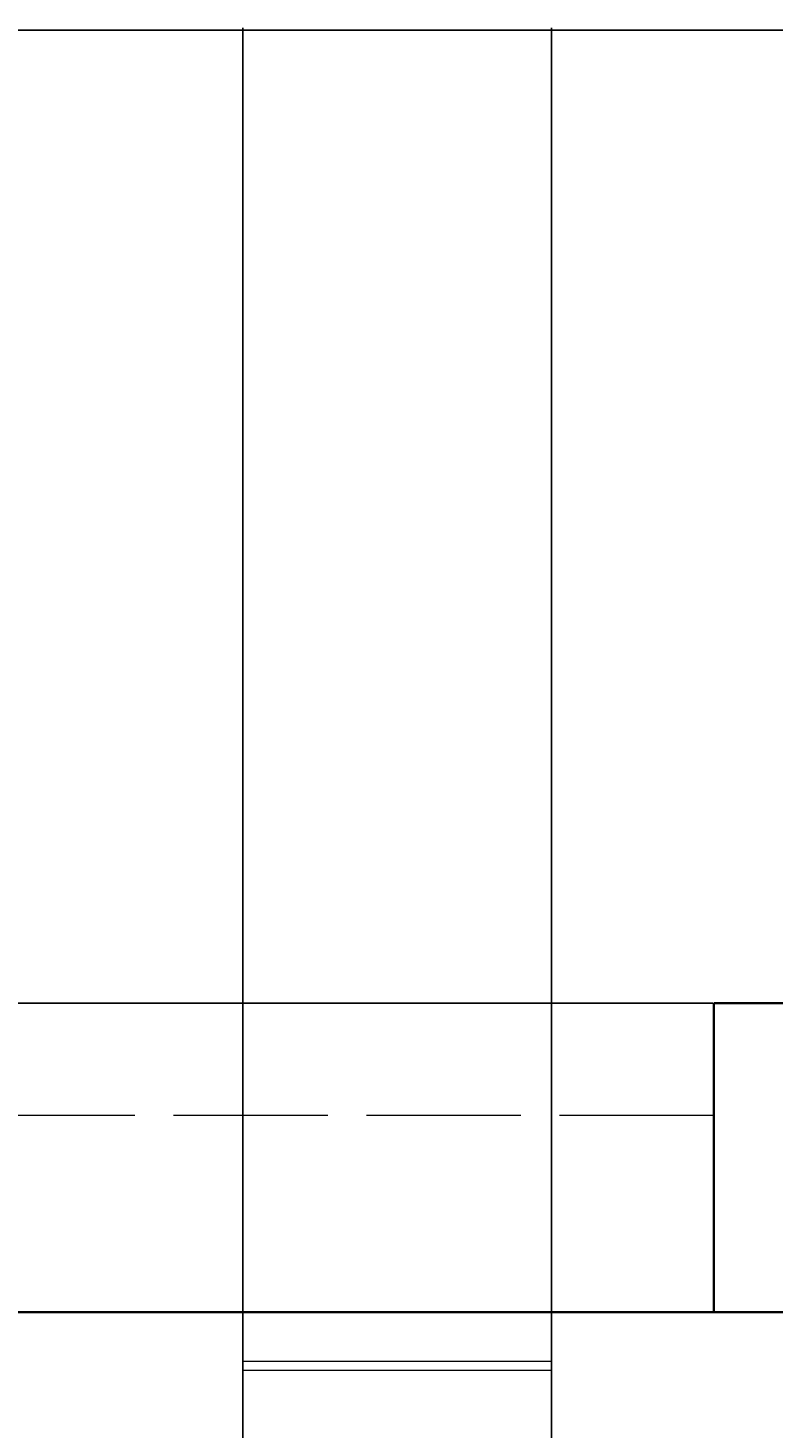
# Model space of a CAD drawing. Units: inches. Extents: x -61 to 1599, y -1316 to 257.
# Tile 142 of 204: x 236 to 294, y 149 to 257. Entities that reach past the tile are written whole.
import ezdxf

# ---------------------------------------------------------------- set-up
doc = ezdxf.new("R2010")
doc.units = ezdxf.units.IN
doc.header["$MEASUREMENT"] = 0
doc.linetypes.add('ACAD_ISO02W100', pattern=[15, 12, -3])
for name, color, linetype, lineweight in [('A-ANNO-DIMS', 2, 'Continuous', 18), ('A-FLOR-OVHD', 203, 'ACAD_ISO02W100', 13), ('WALLS', 4, 'Continuous', 35), ('WINDOWS', 220, 'Continuous', 18)]:
    doc.layers.add(name, color=color, linetype=linetype, lineweight=lineweight)
doc.styles.get("Standard").update_dxf_attribs({"font": 'arial.ttf'})
doc.dimstyles.get("Standard").update_dxf_attribs({"dimtxt": 0.18, "dimasz": 0.18, "dimexe": 0.18, "dimexo": 0.0625, "dimgap": 0.09, "dimtad": 0, "dimtih": 1, "dimtoh": 1, "dimdec": 0, "dimzin": 0, "dimdsep": 46, "dimlunit": 3, "dimtxsty": 'Standard', "dimcen": 0.09, "dimadec": 0, "dimazin": 0, "dimtfac": 1, "dimtdec": 0, "dimtofl": 0, "dimtmove": 0, "dimatfit": 3, "dimfxl": 1, "dimtolj": 1, "dimtzin": 0, "dimarcsym": 0})

# ---------------------------------------------------------------- blocks, each defined once
blk = doc.blocks.new('WIN-24IN')
for p, q in [((0, 4.5), (0, 9)), ((0, 9), (0, 0)), ((24, 9), (24, 0)), ((0, 5.19), (24, 5.19)), ((0, 4.5), (24, 4.5))]:
    blk.add_line(p, q)
blk = doc.blocks.new('*D686')
at = {"layer": 'A-ANNO-DIMS', "color": 0, "lineweight": -2, "transparency": 16777216}
for p, q in [((14.7, 157.74), (14.7, 257.46)), ((14.88, 257.28), (768.35, 257.28)), ((1522.52, 257.28), (769.05, 257.28)), ((1522.7, 157.74), (1522.7, 257.46))]:
    blk.add_line(p, q, dxfattribs=at)
at = {"layer": 'A-ANNO-DIMS', "color": 0, "transparency": 16777216}
for points in [[(14.88, 257.31), (14.88, 257.25), (14.7, 257.28)], [(1522.52, 257.31), (1522.52, 257.25), (1522.7, 257.28)]]:
    blk.add_solid(points, dxfattribs=at)
at = {"layer": 'DEFPOINTS', "color": 0, "transparency": 16777216}
for p in [(1522.7, 257.28), (14.7, 157.68), (1522.7, 157.68)]:
    blk.add_point(p, dxfattribs=at)
at = {"layer": 'A-ANNO-DIMS', "color": 0, "transparency": 16777216, "insert": (768.7, 257.28), "char_height": 0.18, "attachment_point": 5}
blk.add_mtext('\\A1;1508', dxfattribs=at)
blk = doc.blocks.new('*D687')
at = {"layer": 'A-ANNO-DIMS', "color": 0, "lineweight": -2, "transparency": 16777216}
for p, q in [((289.42, 181.68), (-61.08, 181.68)), ((-60.9, 181.5), (-60.9, -528.95)), ((-60.9, -1239.76), (-60.9, -529.32)), ((319.64, -1239.94), (-61.08, -1239.94))]:
    blk.add_line(p, q, dxfattribs=at)
at = {"layer": 'A-ANNO-DIMS', "color": 0, "transparency": 16777216}
for points in [[(-60.93, 181.5), (-60.87, 181.5), (-60.9, 181.68)], [(-60.93, -1239.76), (-60.87, -1239.76), (-60.9, -1239.94)]]:
    blk.add_solid(points, dxfattribs=at)
at = {"layer": 'DEFPOINTS', "color": 0, "transparency": 16777216}
for p in [(289.48, 181.68), (-60.9, -1239.94), (319.7, -1239.94)]:
    blk.add_point(p, dxfattribs=at)
at = {"layer": 'A-ANNO-DIMS', "color": 0, "transparency": 16777216, "insert": (-60.9, -529.13), "char_height": 0.18, "attachment_point": 5}
blk.add_mtext('\\A1;1421.6', dxfattribs=at)
blk = doc.blocks.new('*D701')
at = {"layer": 'A-ANNO-DIMS', "color": 0, "lineweight": -2, "transparency": 16777216}
for p, q in [((215.75, -616.88), (215.75, 257.46)), ((215.93, 257.28), (233.92, 257.28)), ((252.7, 257.28), (234.71, 257.28)), ((252.88, -616.88), (252.88, 257.46))]:
    blk.add_line(p, q, dxfattribs=at)
at = {"layer": 'A-ANNO-DIMS', "color": 0, "transparency": 16777216}
for points in [[(215.93, 257.31), (215.93, 257.25), (215.75, 257.28)], [(252.7, 257.31), (252.7, 257.25), (252.88, 257.28)]]:
    blk.add_solid(points, dxfattribs=at)
at = {"layer": 'DEFPOINTS', "color": 0, "transparency": 16777216}
for p in [(252.88, 257.28), (215.75, -616.94), (252.88, -616.94)]:
    blk.add_point(p, dxfattribs=at)
at = {"layer": 'A-ANNO-DIMS', "color": 0, "transparency": 16777216, "insert": (234.32, 257.28), "char_height": 0.18, "attachment_point": 5}
blk.add_mtext('\\A1;37.13', dxfattribs=at)
blk = doc.blocks.new('*D702')
at = {"layer": 'A-ANNO-DIMS', "color": 0, "lineweight": -2, "transparency": 16777216}
for p, q in [((276.88, -616.88), (276.88, 257.46)), ((277.06, 257.28), (312.21, 257.28)), ((348.14, 257.28), (312.99, 257.28)), ((348.32, -616.88), (348.32, 257.46))]:
    blk.add_line(p, q, dxfattribs=at)
at = {"layer": 'A-ANNO-DIMS', "color": 0, "transparency": 16777216}
for points in [[(277.06, 257.31), (277.06, 257.25), (276.88, 257.28)], [(348.14, 257.31), (348.14, 257.25), (348.32, 257.28)]]:
    blk.add_solid(points, dxfattribs=at)
at = {"layer": 'DEFPOINTS', "color": 0, "transparency": 16777216}
for p in [(348.32, 257.28), (276.88, -616.94), (348.32, -616.94)]:
    blk.add_point(p, dxfattribs=at)
at = {"layer": 'A-ANNO-DIMS', "color": 0, "transparency": 16777216, "insert": (312.6, 257.28), "char_height": 0.18, "attachment_point": 5}
blk.add_mtext('\\A1;71.44', dxfattribs=at)

msp = doc.modelspace()

# ---------------------------------------------------------------- linework, layer by layer
at = {"layer": 'A-FLOR-OVHD'}
msp.add_line((289.4807, 172.9695), (160.8585, 172.9695), dxfattribs=at)
at = {"layer": 'WALLS'}
for p, q in [((289.4807, 157.6771), (289.4807, 181.6771)), ((403.7028, 181.6771), (289.4807, 181.6771)), ((544.7028, 157.6771), (14.7028, 157.6771))]:
    msp.add_line(p, q, dxfattribs=at)

# ---------------------------------------------------------------- block references
at = {"layer": 'WINDOWS'}
msp.add_blockref('WIN-24IN', (252.882, 148.677), dxfattribs=at)

# ---------------------------------------------------------------- dimensions: what is measured, and where the dimension line sits
at = {"layer": 'A-ANNO-DIMS'}
for base, p1, p2, override, picture, middle in [((1522.7028, 257.2771), (14.7028, 157.6771), (1522.7028, 157.6771), {"dimdec": 0, "dimlfac": 1, "dimrnd": 0, "dimzin": 0, "dimdsep": 46, "dimlunit": 2}, '*D686', (768.7028, 257.2771)), ((252.8825, 257.2771), (215.7521, -616.9446), (252.8825, -616.9446), {"dimdec": 2, "dimlfac": 1, "dimrnd": 0, "dimzin": 0, "dimdsep": 46, "dimlunit": 2}, '*D701', (234.3173, 257.2771)), ((348.3201, 257.2771), (276.8825, -616.9446), (348.3201, -616.9446), {"dimdec": 2, "dimlfac": 1, "dimrnd": 0, "dimzin": 0, "dimdsep": 46, "dimlunit": 2}, '*D702', (312.6013, 257.2771))]:
    dim = msp.add_linear_dim(base=base, p1=p1, p2=p2, dimstyle='Standard', override=override, dxfattribs=at)
    dim.commit()
    dim.dimension.update_dxf_attribs({"geometry": picture, "text_midpoint": middle})
dim = msp.add_linear_dim(base=(-60.8972, -1239.9446), p1=(289.4807, 181.6771), p2=(319.7028, -1239.9446), angle=90, dimstyle='Standard', override={"dimdec": 1, "dimlfac": 1, "dimrnd": 0, "dimzin": 0, "dimdsep": 46, "dimlunit": 2}, dxfattribs=at)
dim.commit()
dim.dimension.update_dxf_attribs({"geometry": '*D687', "text_midpoint": (-60.8972, -529.1337)})

doc.saveas('drawing.dxf')
